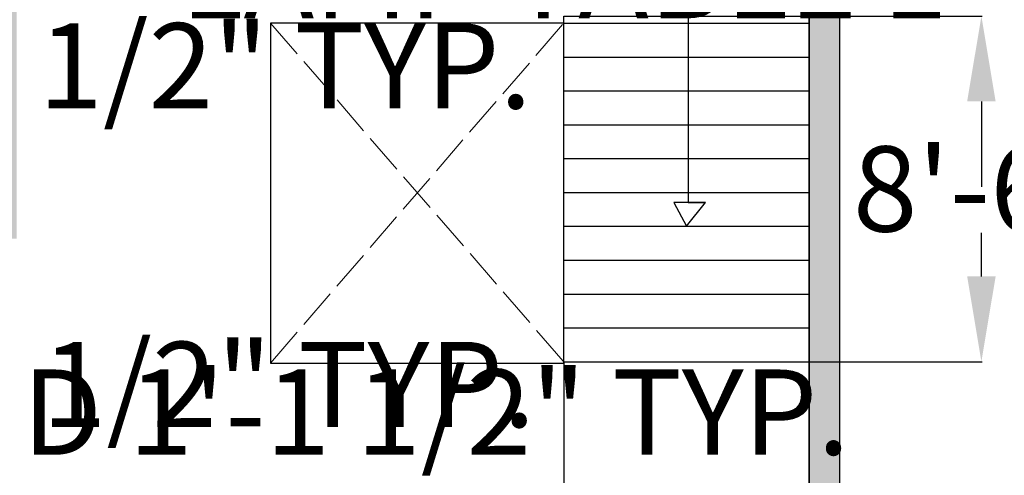
# Model space of a CAD drawing. Units: inches. Extents: x 23 to 3024, y 4 to 1405.
# Tile 5 of 7: x 2558 to 2849, y 955 to 1090. Entities that reach past the tile are written whole.
import ezdxf

# ---------------------------------------------------------------- set-up
doc = ezdxf.new("R2010")
doc.units = ezdxf.units.IN
doc.header["$MEASUREMENT"] = 0
doc.linetypes.add('ACAD_ISO02W100', pattern=[15, 12, -3])
for name, color, linetype, lineweight in [('A-ANNO-DIMS', 2, 'Continuous', 18), ('A-FLOR-STRS', 7, 'Continuous', 25), ('A-FLOR-STRS-OVHD', 8, 'ACAD_ISO02W100', 13), ('A-WALL', 7, 'Continuous', 35), ('A-WALL-PATT', 189, 'Continuous', 13), ('C-PROP', 7, 'Continuous', 30)]:
    doc.layers.add(name, color=color, linetype=linetype, lineweight=lineweight)
doc.styles.get("Standard").update_dxf_attribs({"font": 'arial.ttf'})
doc.dimstyles.get("Standard").update_dxf_attribs({"dimtxt": 25.18, "dimasz": 25.18, "dimexe": 0.18, "dimexo": 0.0625, "dimgap": 0.09, "dimtad": 0, "dimtih": 1, "dimtoh": 1, "dimdec": 0, "dimrnd": 10, "dimzin": 0, "dimdsep": 46, "dimlunit": 3, "dimtxsty": 'Standard', "dimcen": 0.09, "dimadec": 0, "dimazin": 0, "dimtfac": 1, "dimtdec": 0, "dimtofl": 0, "dimtmove": 0, "dimatfit": 3, "dimfxl": 1, "dimtolj": 1, "dimtzin": 0, "dimarcsym": 0})

# ---------------------------------------------------------------- blocks, each defined once
blk = doc.blocks.new('*D21')
at = {"layer": 'A-ANNO-DIMS', "color": 0, "lineweight": -2, "transparency": 16777216}
for p, q in [((2449.18, 913.2), (2449.18, 909.84)), ((2470.74, 913.2), (2470.74, 909.84)), ((2424, 910.02), (2398.82, 910.02)), ((2495.92, 910.02), (2521.1, 910.02))]:
    blk.add_line(p, q, dxfattribs=at)
at = {"layer": 'A-ANNO-DIMS', "color": 0, "transparency": 16777216}
for points in [[(2424, 914.22), (2424, 905.83), (2449.18, 910.02)], [(2495.92, 914.22), (2495.92, 905.83), (2470.74, 910.02)]]:
    blk.add_solid(points, dxfattribs=at)
at = {"layer": 'Defpoints', "color": 0, "transparency": 16777216}
for p in [(2449.18, 913.26), (2470.74, 913.26), (2470.74, 910.02)]:
    blk.add_point(p, dxfattribs=at)
at = {"layer": 'A-ANNO-DIMS', "color": 0, "transparency": 16777216, "insert": (2686.74, 910.02), "char_height": 25.18, "attachment_point": 5}
blk.add_mtext('\\A1;CHAIR 1\'-9 1/2" TYP.', dxfattribs=at)
blk = doc.blocks.new('*D22')
at = {"layer": 'A-ANNO-DIMS', "color": 0, "lineweight": -2, "transparency": 16777216}
for p, q in [((2473.98, 956.88), (2473.98, 982.06)), ((2473.98, 982.06), (2499.16, 982.06)), ((2470.81, 931.7), (2474.16, 931.7)), ((2470.81, 913.26), (2474.16, 913.26)), ((2473.98, 888.08), (2473.98, 862.9))]:
    blk.add_line(p, q, dxfattribs=at)
at = {"layer": 'A-ANNO-DIMS', "color": 0, "transparency": 16777216}
for points in [[(2469.78, 956.88), (2478.17, 956.88), (2473.98, 931.7)], [(2469.78, 888.08), (2478.17, 888.08), (2473.98, 913.26)]]:
    blk.add_solid(points, dxfattribs=at)
at = {"layer": 'Defpoints', "color": 0, "transparency": 16777216}
for p in [(2470.74, 931.7), (2473.98, 931.7), (2470.74, 913.26)]:
    blk.add_point(p, dxfattribs=at)
at = {"layer": 'A-ANNO-DIMS', "color": 0, "transparency": 16777216, "insert": (2604.14, 982.06), "char_height": 25.18, "attachment_point": 5}
blk.add_mtext('\\A1;1\'-6 1/2" TYP.', dxfattribs=at)
blk = doc.blocks.new('*D35')
at = {"layer": 'A-ANNO-DIMS', "color": 0, "lineweight": -2, "transparency": 16777216}
for p, q in [((2272.06, 973.9), (2246.88, 973.9)), ((2297.24, 975.85), (2297.24, 973.72)), ((2310.67, 975.85), (2310.67, 973.72)), ((2335.85, 973.9), (2361.03, 973.9))]:
    blk.add_line(p, q, dxfattribs=at)
at = {"layer": 'A-ANNO-DIMS', "color": 0, "transparency": 16777216}
for points in [[(2272.06, 978.09), (2272.06, 969.7), (2297.24, 973.9)], [(2335.85, 978.09), (2335.85, 969.7), (2310.67, 973.9)]]:
    blk.add_solid(points, dxfattribs=at)
at = {"layer": 'Defpoints', "color": 0, "transparency": 16777216}
for p in [(2297.24, 975.91), (2310.67, 975.91), (2310.67, 973.9)]:
    blk.add_point(p, dxfattribs=at)
at = {"layer": 'A-ANNO-DIMS', "color": 0, "transparency": 16777216, "insert": (2585.8, 973.9), "char_height": 25.18, "attachment_point": 5}
blk.add_mtext('\\A1;NIGHTSTAND 1\'-1 1/2" TYP.', dxfattribs=at)
blk = doc.blocks.new('*D37')
at = {"layer": 'A-ANNO-DIMS', "color": 0, "lineweight": -2, "transparency": 16777216}
for p, q in [((2214.42, 1078.46), (2214.42, 1076)), ((2230.01, 1078.46), (2230.01, 1076)), ((2189.24, 1076.18), (2164.06, 1076.18)), ((2255.19, 1076.18), (2280.37, 1076.18))]:
    blk.add_line(p, q, dxfattribs=at)
at = {"layer": 'A-ANNO-DIMS', "color": 0, "transparency": 16777216}
for points in [[(2189.24, 1080.38), (2189.24, 1071.99), (2214.42, 1076.18)], [(2255.19, 1080.38), (2255.19, 1071.99), (2230.01, 1076.18)]]:
    blk.add_solid(points, dxfattribs=at)
at = {"layer": 'Defpoints', "color": 0, "transparency": 16777216}
for p in [(2214.42, 1078.52), (2230.01, 1078.52), (2230.01, 1076.18)]:
    blk.add_point(p, dxfattribs=at)
at = {"layer": 'A-ANNO-DIMS', "color": 0, "transparency": 16777216, "insert": (2499.37, 1076.18), "char_height": 25.18, "attachment_point": 5}
blk.add_mtext('\\A1;LAMP TABLE 1\'-3 1/2" TYP.', dxfattribs=at)
blk = doc.blocks.new('*D39')
at = {"layer": 'A-ANNO-DIMS', "color": 0, "lineweight": -2, "transparency": 16777216}
for p, q in [((2501.85, 1102.79), (2476.67, 1102.79)), ((2527.03, 1099.9), (2527.03, 1102.97)), ((2546.68, 1099.9), (2546.68, 1102.97)), ((2571.86, 1102.79), (2597.04, 1102.79))]:
    blk.add_line(p, q, dxfattribs=at)
at = {"layer": 'A-ANNO-DIMS', "color": 0, "transparency": 16777216}
for points in [[(2501.85, 1106.99), (2501.85, 1098.59), (2527.03, 1102.79)], [(2571.86, 1106.99), (2571.86, 1098.59), (2546.68, 1102.79)]]:
    blk.add_solid(points, dxfattribs=at)
at = {"layer": 'Defpoints', "color": 0, "transparency": 16777216}
for p in [(2546.68, 1102.79), (2527.03, 1099.84), (2546.68, 1099.84)]:
    blk.add_point(p, dxfattribs=at)
at = {"layer": 'A-ANNO-DIMS', "color": 0, "transparency": 16777216, "insert": (2816.04, 1102.79), "char_height": 25.18, "attachment_point": 5}
blk.add_mtext('\\A1;LAMP TABLE 1\'-7 1/2" TYP.', dxfattribs=at)
blk = doc.blocks.new('*D40')
at = {"layer": 'A-ANNO-DIMS', "color": 0, "lineweight": -2, "transparency": 16777216}
for p, q in [((2524.09, 1125.02), (2524.09, 1150.2)), ((2524.09, 1150.2), (2549.27, 1150.2)), ((2526.97, 1099.84), (2523.91, 1099.84)), ((2526.97, 1084.82), (2523.91, 1084.82)), ((2524.09, 1059.64), (2524.09, 1034.46))]:
    blk.add_line(p, q, dxfattribs=at)
at = {"layer": 'A-ANNO-DIMS', "color": 0, "transparency": 16777216}
for points in [[(2519.89, 1125.02), (2528.28, 1125.02), (2524.09, 1099.84)], [(2519.89, 1059.64), (2528.28, 1059.64), (2524.09, 1084.82)]]:
    blk.add_solid(points, dxfattribs=at)
at = {"layer": 'Defpoints', "color": 0, "transparency": 16777216}
for p in [(2524.09, 1099.84), (2527.03, 1099.84), (2527.03, 1084.82)]:
    blk.add_point(p, dxfattribs=at)
at = {"layer": 'A-ANNO-DIMS', "color": 0, "transparency": 16777216, "insert": (2624.91, 1150.2), "char_height": 25.18, "attachment_point": 5}
blk.add_mtext('\\A1;1\'-3" TYP.', dxfattribs=at)
blk = doc.blocks.new('*D45')
at = {"layer": 'A-ANNO-DIMS', "color": 0, "lineweight": -2, "transparency": 16777216}
for p, q in [((2719, 988.72), (2719, 533.9)), ((2791.45, 988.72), (2791.45, 533.9)), ((2744.18, 534.08), (2766.27, 534.08)), ((2791.45, 534.08), (2816.63, 534.08))]:
    blk.add_line(p, q, dxfattribs=at)
at = {"layer": 'A-ANNO-DIMS', "color": 0, "transparency": 16777216}
for points in [[(2744.18, 538.27), (2744.18, 529.88), (2719, 534.08)], [(2766.27, 538.27), (2766.27, 529.88), (2791.45, 534.08)]]:
    blk.add_solid(points, dxfattribs=at)
at = {"layer": 'Defpoints', "color": 0, "transparency": 16777216}
for p in [(2719, 988.78), (2791.45, 988.78), (2791.45, 534.08)]:
    blk.add_point(p, dxfattribs=at)
at = {"layer": 'A-ANNO-DIMS', "color": 0, "transparency": 16777216, "insert": (2879.59, 534.08), "char_height": 25.18, "attachment_point": 5}
blk.add_mtext('\\A1;6\'-0 1/2"', dxfattribs=at)
blk = doc.blocks.new('*D46')
at = {"layer": 'A-ANNO-DIMS', "color": 0, "lineweight": -2, "transparency": 16777216}
for p, q in [((2719.07, 1090.84), (2842.48, 1090.84)), ((2842.3, 1065.66), (2842.3, 1052.75)), ((2842.3, 1013.96), (2842.3, 1026.86)), ((2791.51, 988.78), (2842.48, 988.78))]:
    blk.add_line(p, q, dxfattribs=at)
at = {"layer": 'A-ANNO-DIMS', "color": 0, "transparency": 16777216}
for points in [[(2838.1, 1065.66), (2846.5, 1065.66), (2842.3, 1090.84)], [(2838.1, 1013.96), (2846.5, 1013.96), (2842.3, 988.78)]]:
    blk.add_solid(points, dxfattribs=at)
at = {"layer": 'Defpoints', "color": 0, "transparency": 16777216}
for p in [(2719, 1090.84), (2842.3, 1090.84), (2791.45, 988.78)]:
    blk.add_point(p, dxfattribs=at)
at = {"layer": 'A-ANNO-DIMS', "color": 0, "transparency": 16777216, "insert": (2842.3, 1039.81), "char_height": 25.18, "attachment_point": 5}
blk.add_mtext('\\A1;8\'-6"', dxfattribs=at)
blk = doc.blocks.new('*D47')
at = {"layer": 'A-ANNO-DIMS', "color": 0, "lineweight": -2, "transparency": 16777216}
for p, q in [((2842.3, 1160.11), (2842.3, 1185.29)), ((2719.07, 1134.93), (2842.48, 1134.93)), ((2719.07, 1090.84), (2842.48, 1090.84)), ((2842.3, 1065.66), (2842.3, 1040.48))]:
    blk.add_line(p, q, dxfattribs=at)
at = {"layer": 'A-ANNO-DIMS', "color": 0, "transparency": 16777216}
for points in [[(2838.1, 1160.11), (2846.5, 1160.11), (2842.3, 1134.93)], [(2838.1, 1065.66), (2846.5, 1065.66), (2842.3, 1090.84)]]:
    blk.add_solid(points, dxfattribs=at)
at = {"layer": 'Defpoints', "color": 0, "transparency": 16777216}
for p in [(2719, 1134.93), (2842.3, 1134.93), (2719, 1090.84)]:
    blk.add_point(p, dxfattribs=at)
at = {"layer": 'A-ANNO-DIMS', "color": 0, "transparency": 16777216, "insert": (2842.3, 1112.88), "char_height": 25.18, "attachment_point": 5}
blk.add_mtext('\\A1;3\'-8"', dxfattribs=at)

msp = doc.modelspace()

# ---------------------------------------------------------------- hatches: boundary and pattern name
at = {"layer": 'A-WALL-PATT'}
h = msp.add_hatch(color=256, dxfattribs=at)
h.dxf.hatch_style = 1
h.paths.add_polyline_path([(2209.45, 1233.93), (2200.45, 1233.93), (2200.45, 1160.43), (2209.45, 1160.43), (2209.45, 1167.77), (2209.45, 1202.93), (2306.45, 1202.93), (2306.45, 1208.93), (2300.45, 1208.93), (2209.45, 1208.93)], flags=17)
h.paths.add_polyline_path([(2800.45, 1295.93), (2200.45, 1295.93), (2160.45, 1295.93), (2160.45, 575.93), (2200.45, 575.93), (2228.06, 575.93), (2228.06, 584.93), (2209.45, 584.93), (2209.45, 856.93), (2200.45, 856.93), (2200.45, 581.93), (2166.45, 581.93), (2166.45, 1289.93), (2200.45, 1289.93), (2200.45, 1261.93), (2209.45, 1261.93), (2209.45, 1286.93), (2244.45, 1286.93), (2300.45, 1286.93), (2300.45, 1241.93), (2301.45, 1241.93, -0.017236), (2303.45, 1241.93), (2306.45, 1241.93), (2306.45, 1286.93), (2548.45, 1286.93), (2548.45, 1261.93), (2557.45, 1261.93), (2557.45, 1286.93), (2791.45, 1286.93), (2791.45, 1140.93), (2613.74, 1140.93), (2613.74, 1134.93), (2791.45, 1134.93), (2791.45, 927.1), (2800.45, 927.1)])
h.paths.add_polyline_path([(2166.06, 1284.53), (2166.03, 1284.87), (2166.29, 1284.91), (2166.32, 1284.58)], flags=16)
h.paths.add_polyline_path([(2557.45, 1233.93), (2548.45, 1233.93), (2548.45, 1208.93), (2514.78, 1208.93), (2457.45, 1208.93), (2451.45, 1208.93), (2451.45, 1202.93), (2548.45, 1202.93), (2557.45, 1202.93)], flags=17)
h.paths.add_polyline_path([(2457.45, 1286.93), (2451.45, 1286.93), (2451.45, 1241.93), (2454.45, 1241.93, -0.017236), (2456.45, 1241.93), (2457.45, 1241.93)], flags=17)
h.paths.add_polyline_path([(2419.96, 1208.93), (2378.45, 1208.93), (2378.45, 1286.93), (2372.45, 1286.93), (2372.45, 1208.93), (2352.45, 1208.93), (2352.45, 1202.93), (2419.96, 1202.93)], flags=17)
h.paths.add_polyline_path([(2557.45, 1134.93), (2563.84, 1134.93), (2563.84, 1140.93), (2557.45, 1140.93), (2557.45, 1149.12), (2548.45, 1149.12), (2548.45, 1103.07), (2548.45, 1065.93), (2416.45, 1065.93), (2416.45, 1064.93, -0.014283), (2416.45, 1062.93), (2416.45, 1059.93), (2548.45, 1059.93), (2548.45, 1025.12), (2557.45, 1025.12)], flags=17)
h.paths.add_polyline_path([(2332.45, 1062.93, -0.014283), (2332.45, 1064.93), (2332.45, 1065.93), (2209.45, 1065.93), (2209.45, 1108.43), (2200.45, 1108.43), (2200.45, 1042.43), (2209.45, 1042.43), (2209.45, 1059.93), (2332.45, 1059.93)], flags=17)
h.paths.add_polyline_path([(2332.45, 996.93), (2209.45, 996.93), (2209.45, 1014.43), (2200.45, 1014.43), (2200.45, 952.93), (2209.45, 952.93), (2209.45, 990.93), (2332.45, 990.93), (2332.45, 991.93, -0.014283), (2332.45, 993.93)], flags=17)
h.paths.add_polyline_path([(2209.45, 900.93), (2200.45, 900.93), (2200.45, 856.93), (2209.45, 856.93), (2255.95, 856.93), (2255.95, 862.93), (2209.45, 862.93)], flags=17)
h.paths.add_polyline_path([(2377.45, 823.93), (2374.45, 823.93, -0.017236), (2372.45, 823.93), (2371.45, 823.93), (2371.45, 763.93), (2312.45, 763.93), (2312.45, 791.27), (2312.45, 796.43), (2306.45, 796.43), (2306.45, 757.93), (2436.95, 757.93), (2436.95, 763.93), (2377.45, 763.93)], flags=17)
h.paths.add_polyline_path([(2557.45, 948.81), (2548.45, 948.81), (2548.45, 763.93), (2488.95, 763.93), (2488.95, 757.93), (2560.45, 757.93), (2560.45, 760.93), (2562.45, 760.93), (2562.45, 763.93), (2557.45, 763.93)], flags=17)
h.paths.add_polyline_path([(2377.45, 990.93), (2371.45, 990.93), (2371.45, 862.93), (2306.45, 862.93), (2306.45, 856.93), (2306.45, 824.43), (2312.45, 824.43), (2312.45, 856.93), (2371.45, 856.93), (2377.45, 856.93)], flags=17)
h.paths.add_polyline_path([(2800.45, 875.1), (2791.45, 875.1), (2791.45, 763.93), (2719.93, 763.93), (2719.93, 757.93), (2791.45, 757.93), (2791.45, 584.93), (2338.88, 584.93), (2338.88, 575.93), (2800.45, 575.93)], flags=17)
h.paths.add_polyline_path([(2667.93, 763.93), (2596.45, 763.93), (2596.45, 762.93, -0.014283), (2596.45, 760.93), (2596.45, 757.93), (2667.93, 757.93)], flags=16)

# ---------------------------------------------------------------- linework, layer by layer
at = {"layer": 'A-FLOR-STRS'}
for p, q in [((2755.69, 1112.88), (2755.69, 1038.78)), ((2719, 988.78), (2719, 1090.84)), ((2719, 1088.78), (2791.45, 1088.78)), ((2719, 1078.78), (2791.45, 1078.78)), ((2719, 1068.78), (2791.45, 1068.78)), ((2719, 1058.78), (2791.45, 1058.78)), ((2719, 1048.78), (2791.45, 1048.78)), ((2719, 1038.78), (2791.45, 1038.78)), ((2755.69, 1038.78), (2755.69, 1035.77)), ((2760.83, 1035.77), (2751.52, 1035.77)), ((2751.52, 1035.77), (2755.23, 1028.78)), ((2755.23, 1028.78), (2760.83, 1035.77)), ((2755.69, 1035.77), (2760.83, 1035.77)), ((2719, 1028.78), (2791.45, 1028.78)), ((2719, 1018.78), (2791.45, 1018.78)), ((2719, 1008.78), (2791.45, 1008.78)), ((2719, 998.78), (2791.45, 998.78)), ((2719, 988.78), (2791.45, 988.78))]:
    msp.add_line(p, q, dxfattribs=at)
msp.add_lwpolyline([(2719, 1088.78), (2632.44, 1088.78), (2632.44, 988.39), (2719, 988.39)], close=True, dxfattribs=at)
at = {"layer": 'A-FLOR-STRS-OVHD'}
for p, q in [((2632.44, 988.39), (2719, 1088.78)), ((2632.44, 1088.78), (2719, 988.78))]:
    msp.add_line(p, q, dxfattribs=at)
at = {"layer": 'A-WALL'}
msp.add_line((2791.45, 1134.93), (2791.45, 763.93), dxfattribs=at)
at = {"layer": 'C-PROP'}
msp.add_line((2800.45, 1295.93), (2800.45, 575.93), dxfattribs=at)

# ---------------------------------------------------------------- dimensions: what is measured, and where the dimension line sits
at = {"layer": 'A-ANNO-DIMS'}
for base, p1, p2, text, picture, middle in [((2546.6795, 1102.7891), (2527.0344, 1099.8423), (2546.6795, 1099.8423), 'LAMP TABLE <> TYP.', '*D39', (2816.0374, 1102.7891)), ((2230.01, 1076.18), (2214.42, 1078.52), (2230.01, 1078.52), 'LAMP TABLE <> TYP.', '*D37', (2499.37, 1076.18)), ((2310.67, 973.9), (2297.24, 975.91), (2310.67, 975.91), 'NIGHTSTAND <> TYP.', '*D35', (2585.8, 973.9)), ((2470.74, 910.02), (2449.18, 913.26), (2470.74, 913.26), 'CHAIR <> TYP.', '*D21', (2686.74, 910.02))]:
    dim = msp.add_linear_dim(base=base, p1=p1, p2=p2, text=text, dimstyle='Standard', override={"dimdec": 1, "dimlfac": 1, "dimrnd": 0, "dimzin": 1, "dimdsep": 46, "dimlunit": 4, "dimfrac": 2}, dxfattribs=at)
    dim.commit()
    dim.dimension.update_dxf_attribs({"geometry": picture, "text_midpoint": middle})
for base, p1, p2, picture, middle in [((2524.09, 1099.84), (2527.03, 1084.82), (2527.03, 1099.84), '*D40', (2624.91, 1150.2)), ((2473.98, 931.7), (2470.74, 913.26), (2470.74, 931.7), '*D22', (2604.14, 982.06))]:
    dim = msp.add_linear_dim(base=base, p1=p1, p2=p2, angle=90, text='<> TYP.', dimstyle='Standard', override={"dimdec": 1, "dimlfac": 1, "dimrnd": 0, "dimzin": 1, "dimdsep": 46, "dimlunit": 4, "dimfrac": 2}, dxfattribs=at)
    dim.commit()
    dim.dimension.update_dxf_attribs({"geometry": picture, "text_midpoint": middle})
for base, p1, p2, picture, middle in [((2842.3, 1134.93), (2719, 1090.84), (2719, 1134.93), '*D47', (2842.3, 1112.88)), ((2842.3, 1090.84), (2791.45, 988.78), (2719, 1090.84), '*D46', (2842.3, 1039.81))]:
    dim = msp.add_linear_dim(base=base, p1=p1, p2=p2, angle=90, dimstyle='Standard', override={"dimdec": 1, "dimlfac": 1, "dimrnd": 0, "dimzin": 1, "dimdsep": 46, "dimlunit": 4, "dimfrac": 2}, dxfattribs=at)
    dim.commit()
    dim.dimension.update_dxf_attribs({"geometry": picture, "text_midpoint": middle})
dim = msp.add_linear_dim(base=(2791.449, 534.0772), p1=(2719.0035, 988.7789), p2=(2791.449, 988.7789), dimstyle='Standard', override={"dimdec": 1, "dimlfac": 1, "dimrnd": 0, "dimzin": 1, "dimdsep": 46, "dimlunit": 4, "dimfrac": 2}, dxfattribs=at)
dim.commit()
dim.dimension.update_dxf_attribs({"geometry": '*D45', "text_midpoint": (2879.5917, 534.0772)})

doc.saveas('drawing.dxf')
